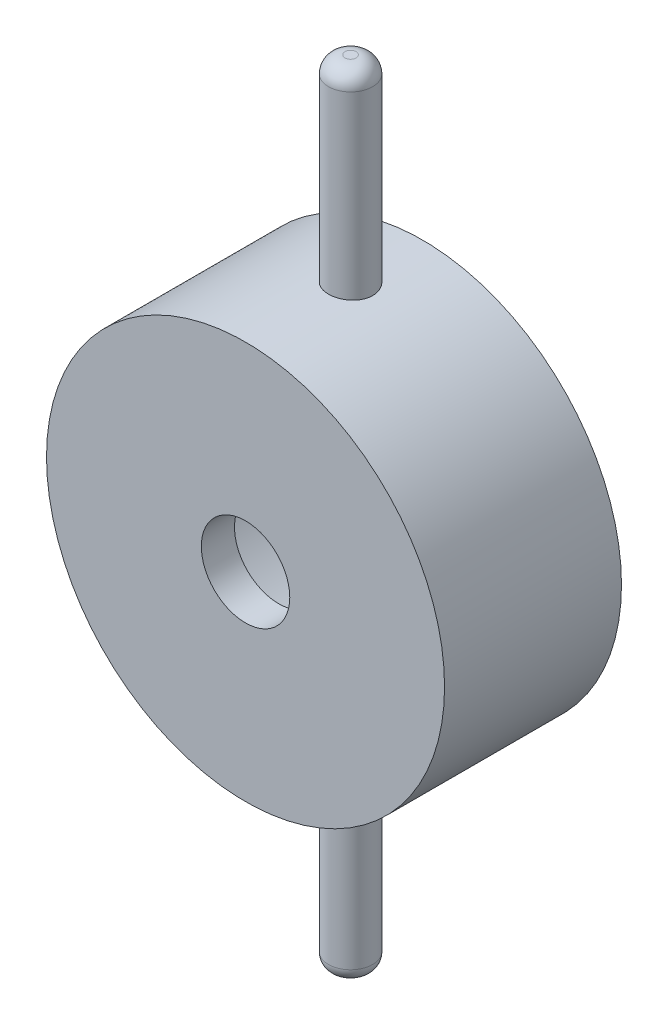
ISO-10303-21;
HEADER;
FILE_DESCRIPTION(('STEP AP214'),'2;1');
FILE_NAME('part.step','',(''),(''),'','','');
FILE_SCHEMA(('AUTOMOTIVE_DESIGN { 1 0 10303 214 1 1 1 1 }'));
ENDSEC;
DATA;
#1=APPLICATION_CONTEXT('core data for automotive mechanical design processes');
#2=APPLICATION_PROTOCOL_DEFINITION('international standard','automotive_design',2000,#1);
#3=PRODUCT_CONTEXT('',#1,'mechanical');
#4=PRODUCT('Part','Part','',(#3));
#5=PRODUCT_RELATED_PRODUCT_CATEGORY('part','',(#4));
#6=PRODUCT_DEFINITION_FORMATION('','',#4);
#7=PRODUCT_DEFINITION_CONTEXT('part definition',#1,'design');
#8=PRODUCT_DEFINITION('design','',#6,#7);
#9=PRODUCT_DEFINITION_SHAPE('','',#8);
#10=(LENGTH_UNIT() NAMED_UNIT(*) SI_UNIT(.MILLI.,.METRE.));
#11=(NAMED_UNIT(*) PLANE_ANGLE_UNIT() SI_UNIT($,.RADIAN.));
#12=(NAMED_UNIT(*) SI_UNIT($,.STERADIAN.) SOLID_ANGLE_UNIT());
#13=UNCERTAINTY_MEASURE_WITH_UNIT(LENGTH_MEASURE(1.E-05),#10,'distance_accuracy_value','');
#14=(GEOMETRIC_REPRESENTATION_CONTEXT(3) GLOBAL_UNCERTAINTY_ASSIGNED_CONTEXT((#13)) GLOBAL_UNIT_ASSIGNED_CONTEXT((#10,
#11,#12)) REPRESENTATION_CONTEXT('',''));
#15=CARTESIAN_POINT('',(0.,0.,0.));
#16=DIRECTION('',(0.,0.,1.));
#17=DIRECTION('',(1.,0.,0.));
#18=AXIS2_PLACEMENT_3D('',#15,#16,#17);
#19=CARTESIAN_POINT('',(0.,0.,32.));
#20=DIRECTION('',(0.,0.,-1.));
#21=DIRECTION('',(-1.,0.,0.));
#22=AXIS2_PLACEMENT_3D('',#19,#20,#21);
#23=CYLINDRICAL_SURFACE('',#22,36.);
#24=CARTESIAN_POINT('',(0.,-36.,17.));
#25=CARTESIAN_POINT('',(0.223941264699037,-35.9999971710871,16.9999903743455));
#26=CARTESIAN_POINT('',(0.448027205939019,-35.9978882822096,16.9811305097902));
#27=CARTESIAN_POINT('',(0.889976947693404,-35.9896783191239,16.9061849431516));
#28=CARTESIAN_POINT('',(1.10783377823557,-35.983572942543,16.8500591218983));
#29=CARTESIAN_POINT('',(1.53086215814058,-35.9680586147846,16.7022440896357));
#30=CARTESIAN_POINT('',(1.73604164147526,-35.9586517549432,16.6105773882806));
#31=CARTESIAN_POINT('',(2.12806106019971,-35.9375839621738,16.3943287716029));
#32=CARTESIAN_POINT('',(2.31490442346979,-35.9259234517738,16.2697530246617));
#33=CARTESIAN_POINT('',(2.66581151494052,-35.9015954363711,15.9906358997437));
#34=CARTESIAN_POINT('',(2.8297831590842,-35.8889241662728,15.8359790702864));
#35=CARTESIAN_POINT('',(3.12950007420101,-35.8640335665073,15.501337047927));
#36=CARTESIAN_POINT('',(3.26524398598451,-35.8518142586257,15.3213506360829));
#37=CARTESIAN_POINT('',(3.50498603632461,-35.8291733589873,14.9405721435395));
#38=CARTESIAN_POINT('',(3.60889951084678,-35.8187565931509,14.7397264459003));
#39=CARTESIAN_POINT('',(3.78149035601591,-35.8009483607062,14.3233010786259));
#40=CARTESIAN_POINT('',(3.85016879003953,-35.7935568027999,14.107721853864));
#41=CARTESIAN_POINT('',(3.95006388985288,-35.7826708846305,13.6688960042714));
#42=CARTESIAN_POINT('',(3.98143459684434,-35.7791605034939,13.4456848498581));
#43=CARTESIAN_POINT('',(4.00630012007012,-35.7763850132246,12.9971402763398));
#44=CARTESIAN_POINT('',(3.99979615128966,-35.7771197679119,12.7718069255444));
#45=CARTESIAN_POINT('',(3.94922368855802,-35.782736882028,12.3264810500568));
#46=CARTESIAN_POINT('',(3.90532400345945,-35.7876006024619,12.1064690866508));
#47=CARTESIAN_POINT('',(3.78146922315378,-35.8008985434681,11.6769547492225));
#48=CARTESIAN_POINT('',(3.70151353860304,-35.809332822402,11.4674525470469));
#49=CARTESIAN_POINT('',(3.50763212158903,-35.8288428850078,11.0643751536738));
#50=CARTESIAN_POINT('',(3.3936321376296,-35.8399244317603,10.8708359679684));
#51=CARTESIAN_POINT('',(3.13495141327351,-35.8634757446383,10.5055726985383));
#52=CARTESIAN_POINT('',(2.99026956353588,-35.8759455609506,10.3338494039533));
#53=CARTESIAN_POINT('',(2.67339229787913,-35.9009513795857,10.0161120313828));
#54=CARTESIAN_POINT('',(2.50105121133653,-35.9134873721861,9.87024318955051));
#55=CARTESIAN_POINT('',(2.13425163992195,-35.9371491420364,9.60948323665533));
#56=CARTESIAN_POINT('',(1.93979312055407,-35.9482749170867,9.49459217390847));
#57=CARTESIAN_POINT('',(1.53417327107101,-35.9678676205184,9.29905247047048));
#58=CARTESIAN_POINT('',(1.32300800960341,-35.976333920741,9.21841191804988));
#59=CARTESIAN_POINT('',(0.890019511278724,-35.9896476900257,9.09377244991667));
#60=CARTESIAN_POINT('',(0.668196668515817,-35.99449529279,9.04977218042734));
#61=CARTESIAN_POINT('',(0.221446663788539,-36.0000082213112,8.99984819656494));
#62=CARTESIAN_POINT('',(-0.00345785778178484,-36.0006955440179,8.99372421240759));
#63=CARTESIAN_POINT('',(-0.451089977374322,-35.997869624086,9.01919958502613));
#64=CARTESIAN_POINT('',(-0.67381761178264,-35.9943564517791,9.05079831018584));
#65=CARTESIAN_POINT('',(-1.11019011884666,-35.9835381866102,9.1506558809117));
#66=CARTESIAN_POINT('',(-1.32385687712367,-35.9762428689165,9.21882023623495));
#67=CARTESIAN_POINT('',(-1.73672454025379,-35.9586780068327,9.38977655545623));
#68=CARTESIAN_POINT('',(-1.93592504958459,-35.9484083811602,9.49256946570207));
#69=CARTESIAN_POINT('',(-2.31510653023491,-35.9259871400455,9.73035658214195));
#70=CARTESIAN_POINT('',(-2.49500506278204,-35.9138279560722,9.86548152187963));
#71=CARTESIAN_POINT('',(-2.82963966960439,-35.8890143170873,10.1639105966687));
#72=CARTESIAN_POINT('',(-2.98437496031115,-35.876359846668,10.3272156089047));
#73=CARTESIAN_POINT('',(-3.26499244865632,-35.851914968072,10.6782465781321));
#74=CARTESIAN_POINT('',(-3.39074265075841,-35.840128672854,10.8660783809566));
#75=CARTESIAN_POINT('',(-3.60891112010016,-35.8188194574623,11.2603125669849));
#76=CARTESIAN_POINT('',(-3.70132993400149,-35.809296500169,11.4667146455518));
#77=CARTESIAN_POINT('',(-3.84999424202287,-35.7936189645329,11.8917889174332));
#78=CARTESIAN_POINT('',(-3.90631654962256,-35.787457237671,12.1104339714952));
#79=CARTESIAN_POINT('',(-3.98143755533594,-35.7791783914912,12.5541502954833));
#80=CARTESIAN_POINT('',(-4.00023760641309,-35.7770611263396,12.7792213334069));
#81=CARTESIAN_POINT('',(-3.99975914683357,-35.7771145169331,13.2280883101301));
#82=CARTESIAN_POINT('',(-3.98068798086116,-35.7792618241774,13.4518845013619));
#83=CARTESIAN_POINT('',(-3.9054450016096,-35.7875524591414,13.8930714766512));
#84=CARTESIAN_POINT('',(-3.84927316073427,-35.7936957898334,14.1104622559441));
#85=CARTESIAN_POINT('',(-3.70148382525128,-35.8092794902223,14.5326550210184));
#86=CARTESIAN_POINT('',(-3.60987407876389,-35.8187191391705,14.7374597472708));
#87=CARTESIAN_POINT('',(-3.39383017574505,-35.8398332240413,15.1288209868962));
#88=CARTESIAN_POINT('',(-3.26939595247519,-35.8515076645075,15.3153774631659));
#89=CARTESIAN_POINT('',(-2.99045990507415,-35.8758525588044,15.6660084922529));
#90=CARTESIAN_POINT('',(-2.83580341800636,-35.888527927148,15.8299596709519));
#91=CARTESIAN_POINT('',(-2.50112838496826,-35.9134021228346,16.1296677444216));
#92=CARTESIAN_POINT('',(-2.32110381521302,-35.925600836112,16.2654179237183));
#93=CARTESIAN_POINT('',(-1.94018897354974,-35.9481870419338,16.5052086607003));
#94=CARTESIAN_POINT('',(-1.73923689283218,-35.9585689117416,16.6091514994619));
#95=CARTESIAN_POINT('',(-1.32273699032246,-35.9762927086713,16.7816749848897));
#96=CARTESIAN_POINT('',(-1.10720567988888,-35.9836380098711,16.8502949014684));
#97=CARTESIAN_POINT('',(-0.742080478625196,-35.9926465105181,16.9333983229315));
#98=CARTESIAN_POINT('',(-0.594808269722724,-35.9953909720073,16.9583390968784));
#99=CARTESIAN_POINT('',(-0.298378779805415,-35.9990686543792,16.991643097728));
#100=CARTESIAN_POINT('',(-0.149221508955014,-36.0000018850239,17.0000064139796));
#101=CARTESIAN_POINT('',(0.,-36.,17.));
#102=B_SPLINE_CURVE_WITH_KNOTS('',3,(#24,#25,#26,#27,#28,#29,#30,#31,#32,#33,#34,#35,#36,#37,
#38,#39,#40,#41,#42,#43,#44,#45,#46,#47,#48,#49,#50,#51,#52,#53,#54,#55,#56,#57,#58,#59,#60,#61,
#62,#63,#64,#65,#66,#67,#68,#69,#70,#71,#72,#73,#74,#75,#76,#77,#78,#79,#80,#81,#82,#83,#84,#85,
#86,#87,#88,#89,#90,#91,#92,#93,#94,#95,#96,#97,#98,#99,#100,#101),.UNSPECIFIED.,.T.,.F.,(4,2,2,
2,2,2,2,2,2,2,2,2,2,2,2,2,2,2,2,2,2,2,2,2,2,2,2,2,2,2,2,2,2,2,2,2,2,2,4),(0.,0.671278828541613,
1.34328150567798,2.01485926640149,2.68631123763438,3.36039299568731,4.03450720384592,
4.71039918612456,5.38627076910675,6.05934192440493,6.73239148831025,7.40241882686268,
8.07245711756367,8.74396758666022,9.41550233919238,10.0906974506658,10.7658936152352,
11.4412491390922,12.1165797089621,12.7883364134081,13.4600818703464,14.1300997551881,
14.8001359521254,15.4729286177529,16.1457422297356,16.8215617711571,17.4973702280883,
18.1717357450427,18.8460769455389,19.5167363107972,20.1873961749054,20.8579094891852,
21.5284241667564,22.2024645893278,22.8766653369059,23.5529170457317,24.2284153057591,
24.675719109969,25.1230205033015),.UNSPECIFIED.);
#103=CARTESIAN_POINT('',(0.,-36.,17.));
#104=VERTEX_POINT('',#103);
#105=EDGE_CURVE('E54',#104,#104,#102,.T.);
#106=ORIENTED_EDGE('',*,*,#105,.T.);
#107=EDGE_LOOP('',(#106));
#108=FACE_BOUND('',#107,.T.);
#109=CARTESIAN_POINT('',(0.,0.,32.));
#110=DIRECTION('',(0.,0.,1.));
#111=DIRECTION('',(1.,0.,0.));
#112=AXIS2_PLACEMENT_3D('',#109,#110,#111);
#113=CIRCLE('',#112,36.);
#114=CARTESIAN_POINT('',(36.,0.,32.));
#115=VERTEX_POINT('',#114);
#116=EDGE_CURVE('E95',#115,#115,#113,.T.);
#117=ORIENTED_EDGE('',*,*,#116,.F.);
#118=EDGE_LOOP('',(#117));
#119=FACE_BOUND('',#118,.T.);
#120=CARTESIAN_POINT('',(0.,0.,0.));
#121=DIRECTION('',(0.,0.,1.));
#122=DIRECTION('',(1.,0.,0.));
#123=AXIS2_PLACEMENT_3D('',#120,#121,#122);
#124=CIRCLE('',#123,36.);
#125=CARTESIAN_POINT('',(36.,0.,0.));
#126=VERTEX_POINT('',#125);
#127=EDGE_CURVE('E65',#126,#126,#124,.T.);
#128=ORIENTED_EDGE('',*,*,#127,.T.);
#129=EDGE_LOOP('',(#128));
#130=FACE_BOUND('',#129,.T.);
#131=CARTESIAN_POINT('',(0.,36.,9.));
#132=CARTESIAN_POINT('',(-0.223941264699037,35.9999971710871,9.00000962565452));
#133=CARTESIAN_POINT('',(-0.448027205939019,35.9978882822096,9.01886949020976));
#134=CARTESIAN_POINT('',(-0.889976947693403,35.9896783191239,9.09381505684837));
#135=CARTESIAN_POINT('',(-1.10783377823557,35.983572942543,9.14994087810168));
#136=CARTESIAN_POINT('',(-1.53086215814058,35.9680586147846,9.29775591036431));
#137=CARTESIAN_POINT('',(-1.73604164147526,35.9586517549432,9.38942261171939));
#138=CARTESIAN_POINT('',(-2.12806106019971,35.9375839621738,9.60567122839708));
#139=CARTESIAN_POINT('',(-2.31490442346979,35.9259234517738,9.73024697533831));
#140=CARTESIAN_POINT('',(-2.66581151494052,35.9015954363711,10.0093641002563));
#141=CARTESIAN_POINT('',(-2.8297831590842,35.8889241662728,10.1640209297136));
#142=CARTESIAN_POINT('',(-3.12950007420101,35.8640335665073,10.498662952073));
#143=CARTESIAN_POINT('',(-3.26524398598451,35.8518142586257,10.6786493639171));
#144=CARTESIAN_POINT('',(-3.5049860363246,35.8291733589873,11.0594278564605));
#145=CARTESIAN_POINT('',(-3.60889951084678,35.8187565931509,11.2602735540997));
#146=CARTESIAN_POINT('',(-3.78149035601591,35.8009483607062,11.6766989213741));
#147=CARTESIAN_POINT('',(-3.85016879003952,35.7935568027999,11.892278146136));
#148=CARTESIAN_POINT('',(-3.95006388985288,35.7826708846305,12.3311039957286));
#149=CARTESIAN_POINT('',(-3.98143459684434,35.7791605034939,12.5543151501419));
#150=CARTESIAN_POINT('',(-4.00630012007012,35.7763850132246,13.0028597236602));
#151=CARTESIAN_POINT('',(-3.99979615128966,35.7771197679119,13.2281930744555));
#152=CARTESIAN_POINT('',(-3.94922368855802,35.782736882028,13.6735189499432));
#153=CARTESIAN_POINT('',(-3.90532400345945,35.7876006024619,13.8935309133492));
#154=CARTESIAN_POINT('',(-3.78146922315378,35.8008985434681,14.3230452507775));
#155=CARTESIAN_POINT('',(-3.70151353860304,35.809332822402,14.5325474529531));
#156=CARTESIAN_POINT('',(-3.50763212158903,35.8288428850078,14.9356248463262));
#157=CARTESIAN_POINT('',(-3.3936321376296,35.8399244317603,15.1291640320316));
#158=CARTESIAN_POINT('',(-3.1349514132735,35.8634757446383,15.4944273014617));
#159=CARTESIAN_POINT('',(-2.99026956353588,35.8759455609506,15.6661505960467));
#160=CARTESIAN_POINT('',(-2.67339229787913,35.9009513795857,15.9838879686172));
#161=CARTESIAN_POINT('',(-2.50105121133653,35.9134873721861,16.1297568104495));
#162=CARTESIAN_POINT('',(-2.13425163992195,35.9371491420364,16.3905167633447));
#163=CARTESIAN_POINT('',(-1.93979312055407,35.9482749170867,16.5054078260915));
#164=CARTESIAN_POINT('',(-1.53417327107101,35.9678676205184,16.7009475295295));
#165=CARTESIAN_POINT('',(-1.32300800960341,35.976333920741,16.7815880819501));
#166=CARTESIAN_POINT('',(-0.890019511278724,35.9896476900257,16.9062275500833));
#167=CARTESIAN_POINT('',(-0.668196668515818,35.99449529279,16.9502278195727));
#168=CARTESIAN_POINT('',(-0.22144666378854,36.0000082213112,17.0001518034351));
#169=CARTESIAN_POINT('',(0.00345785778178408,36.0006955440179,17.0062757875924));
#170=CARTESIAN_POINT('',(0.451089977374321,35.997869624086,16.9808004149739));
#171=CARTESIAN_POINT('',(0.673817611782639,35.9943564517791,16.9492016898142));
#172=CARTESIAN_POINT('',(1.11019011884666,35.9835381866102,16.8493441190883));
#173=CARTESIAN_POINT('',(1.32385687712367,35.9762428689165,16.781179763765));
#174=CARTESIAN_POINT('',(1.73672454025379,35.9586780068327,16.6102234445438));
#175=CARTESIAN_POINT('',(1.93592504958458,35.9484083811602,16.5074305342979));
#176=CARTESIAN_POINT('',(2.31510653023491,35.9259871400455,16.269643417858));
#177=CARTESIAN_POINT('',(2.49500506278204,35.9138279560722,16.1345184781204));
#178=CARTESIAN_POINT('',(2.82963966960439,35.8890143170873,15.8360894033313));
#179=CARTESIAN_POINT('',(2.98437496031115,35.876359846668,15.6727843910953));
#180=CARTESIAN_POINT('',(3.26499244865632,35.851914968072,15.3217534218679));
#181=CARTESIAN_POINT('',(3.39074265075841,35.840128672854,15.1339216190434));
#182=CARTESIAN_POINT('',(3.60891112010016,35.8188194574623,14.7396874330151));
#183=CARTESIAN_POINT('',(3.70132993400149,35.809296500169,14.5332853544482));
#184=CARTESIAN_POINT('',(3.84999424202287,35.7936189645329,14.1082110825668));
#185=CARTESIAN_POINT('',(3.90631654962256,35.787457237671,13.8895660285048));
#186=CARTESIAN_POINT('',(3.98143755533594,35.7791783914912,13.4458497045167));
#187=CARTESIAN_POINT('',(4.00023760641309,35.7770611263396,13.2207786665931));
#188=CARTESIAN_POINT('',(3.99975914683357,35.7771145169331,12.7719116898699));
#189=CARTESIAN_POINT('',(3.98068798086116,35.7792618241774,12.5481154986381));
#190=CARTESIAN_POINT('',(3.9054450016096,35.7875524591414,12.1069285233488));
#191=CARTESIAN_POINT('',(3.84927316073427,35.7936957898334,11.8895377440559));
#192=CARTESIAN_POINT('',(3.70148382525128,35.8092794902223,11.4673449789816));
#193=CARTESIAN_POINT('',(3.60987407876389,35.8187191391705,11.2625402527292));
#194=CARTESIAN_POINT('',(3.39383017574505,35.8398332240413,10.8711790131038));
#195=CARTESIAN_POINT('',(3.26939595247519,35.8515076645075,10.6846225368341));
#196=CARTESIAN_POINT('',(2.99045990507415,35.8758525588044,10.3339915077471));
#197=CARTESIAN_POINT('',(2.83580341800636,35.888527927148,10.1700403290481));
#198=CARTESIAN_POINT('',(2.50112838496826,35.9134021228346,9.8703322555784));
#199=CARTESIAN_POINT('',(2.32110381521302,35.925600836112,9.73458207628167));
#200=CARTESIAN_POINT('',(1.94018897354974,35.9481870419338,9.49479133929974));
#201=CARTESIAN_POINT('',(1.73923689283218,35.9585689117416,9.39084850053812));
#202=CARTESIAN_POINT('',(1.32273699032246,35.9762927086713,9.21832501511034));
#203=CARTESIAN_POINT('',(1.10720567988888,35.9836380098711,9.14970509853163));
#204=CARTESIAN_POINT('',(0.742080478625197,35.9926465105181,9.06660167706846));
#205=CARTESIAN_POINT('',(0.594808269722725,35.9953909720073,9.04166090312157));
#206=CARTESIAN_POINT('',(0.298378779805415,35.9990686543792,9.00835690227201));
#207=CARTESIAN_POINT('',(0.149221508955014,36.0000018850239,8.99999358602045));
#208=CARTESIAN_POINT('',(0.,36.,9.));
#209=B_SPLINE_CURVE_WITH_KNOTS('',3,(#131,#132,#133,#134,#135,#136,#137,#138,#139,#140,#141,
#142,#143,#144,#145,#146,#147,#148,#149,#150,#151,#152,#153,#154,#155,#156,#157,#158,#159,#160,
#161,#162,#163,#164,#165,#166,#167,#168,#169,#170,#171,#172,#173,#174,#175,#176,#177,#178,#179,
#180,#181,#182,#183,#184,#185,#186,#187,#188,#189,#190,#191,#192,#193,#194,#195,#196,#197,#198,
#199,#200,#201,#202,#203,#204,#205,#206,#207,#208),.UNSPECIFIED.,.T.,.F.,(4,2,2,2,2,2,2,2,2,2,2,
2,2,2,2,2,2,2,2,2,2,2,2,2,2,2,2,2,2,2,2,2,2,2,2,2,2,2,4),(0.,0.671278828541613,1.34328150567797,
2.01485926640149,2.68631123763438,3.3603929956873,4.03450720384592,4.71039918612456,
5.38627076910675,6.05934192440493,6.73239148831025,7.40241882686268,8.07245711756367,
8.74396758666022,9.41550233919238,10.0906974506658,10.7658936152352,11.4412491390922,
12.1165797089621,12.7883364134081,13.4600818703464,14.1300997551881,14.8001359521254,
15.4729286177529,16.1457422297356,16.8215617711571,17.4973702280883,18.1717357450427,
18.8460769455388,19.5167363107972,20.1873961749054,20.8579094891852,21.5284241667564,
22.2024645893278,22.8766653369059,23.5529170457317,24.2284153057591,24.675719109969,
25.1230205033015),.UNSPECIFIED.);
#210=CARTESIAN_POINT('',(0.,36.,9.));
#211=VERTEX_POINT('',#210);
#212=EDGE_CURVE('E86',#211,#211,#209,.T.);
#213=ORIENTED_EDGE('',*,*,#212,.F.);
#214=EDGE_LOOP('',(#213));
#215=FACE_BOUND('',#214,.T.);
#216=ADVANCED_FACE('F40',(#108,#119,#130,#215),#23,.T.);
#217=CARTESIAN_POINT('',(0.,0.,32.));
#218=DIRECTION('',(0.,0.,1.));
#219=DIRECTION('',(1.,0.,0.));
#220=AXIS2_PLACEMENT_3D('',#217,#218,#219);
#221=PLANE('',#220);
#222=CARTESIAN_POINT('',(0.,0.,32.));
#223=DIRECTION('',(0.,0.,1.));
#224=DIRECTION('',(1.,0.,0.));
#225=AXIS2_PLACEMENT_3D('',#222,#223,#224);
#226=CIRCLE('',#225,8.);
#227=CARTESIAN_POINT('',(8.,0.,32.));
#228=VERTEX_POINT('',#227);
#229=EDGE_CURVE('E132',#228,#228,#226,.T.);
#230=ORIENTED_EDGE('',*,*,#229,.F.);
#231=EDGE_LOOP('',(#230));
#232=FACE_BOUND('',#231,.T.);
#233=ORIENTED_EDGE('',*,*,#116,.T.);
#234=EDGE_LOOP('',(#233));
#235=FACE_BOUND('',#234,.T.);
#236=ADVANCED_FACE('F83',(#232,#235),#221,.T.);
#237=CARTESIAN_POINT('',(0.,0.,0.));
#238=DIRECTION('',(0.,0.,1.));
#239=DIRECTION('',(1.,0.,0.));
#240=AXIS2_PLACEMENT_3D('',#237,#238,#239);
#241=PLANE('',#240);
#242=CARTESIAN_POINT('',(0.,0.,0.));
#243=DIRECTION('',(0.,0.,-1.));
#244=DIRECTION('',(-1.,0.,0.));
#245=AXIS2_PLACEMENT_3D('',#242,#243,#244);
#246=CIRCLE('',#245,28.);
#247=CARTESIAN_POINT('',(-28.,0.,0.));
#248=VERTEX_POINT('',#247);
#249=EDGE_CURVE('E134',#248,#248,#246,.T.);
#250=ORIENTED_EDGE('',*,*,#249,.F.);
#251=EDGE_LOOP('',(#250));
#252=FACE_BOUND('',#251,.T.);
#253=ORIENTED_EDGE('',*,*,#127,.F.);
#254=EDGE_LOOP('',(#253));
#255=FACE_BOUND('',#254,.T.);
#256=ADVANCED_FACE('F84',(#252,#255),#241,.F.);
#257=CARTESIAN_POINT('',(0.,71.5,13.));
#258=DIRECTION('',(0.,-1.,0.));
#259=DIRECTION('',(0.,0.,-1.));
#260=AXIS2_PLACEMENT_3D('',#257,#258,#259);
#261=CYLINDRICAL_SURFACE('',#260,4.);
#262=CARTESIAN_POINT('',(0.,68.5,13.));
#263=DIRECTION('',(0.,1.,0.));
#264=DIRECTION('',(0.,0.,1.));
#265=AXIS2_PLACEMENT_3D('',#262,#263,#264);
#266=CIRCLE('',#265,4.);
#267=CARTESIAN_POINT('',(0.,68.5,17.));
#268=VERTEX_POINT('',#267);
#269=EDGE_CURVE('E48',#268,#268,#266,.F.);
#270=ORIENTED_EDGE('',*,*,#269,.T.);
#271=EDGE_LOOP('',(#270));
#272=FACE_BOUND('',#271,.T.);
#273=ORIENTED_EDGE('',*,*,#212,.T.);
#274=EDGE_LOOP('',(#273));
#275=FACE_BOUND('',#274,.T.);
#276=ADVANCED_FACE('F76',(#272,#275),#261,.T.);
#277=CARTESIAN_POINT('',(0.,71.5,13.));
#278=DIRECTION('',(0.,1.,0.));
#279=DIRECTION('',(0.,0.,1.));
#280=AXIS2_PLACEMENT_3D('',#277,#278,#279);
#281=PLANE('',#280);
#282=CARTESIAN_POINT('',(0.,71.5,13.));
#283=DIRECTION('',(0.,1.,0.));
#284=DIRECTION('',(0.,0.,1.));
#285=AXIS2_PLACEMENT_3D('',#282,#283,#284);
#286=CIRCLE('',#285,1.);
#287=CARTESIAN_POINT('',(0.,71.5,14.));
#288=VERTEX_POINT('',#287);
#289=EDGE_CURVE('E55',#288,#288,#286,.T.);
#290=ORIENTED_EDGE('',*,*,#289,.T.);
#291=EDGE_LOOP('',(#290));
#292=FACE_BOUND('',#291,.T.);
#293=ADVANCED_FACE('F72',(#292),#281,.T.);
#294=CARTESIAN_POINT('',(0.,68.5,13.));
#295=DIRECTION('',(0.,1.,0.));
#296=DIRECTION('',(0.,0.,1.));
#297=AXIS2_PLACEMENT_3D('',#294,#295,#296);
#298=DEGENERATE_TOROIDAL_SURFACE('',#297,1.,3.,.T.);
#299=ORIENTED_EDGE('',*,*,#269,.F.);
#300=EDGE_LOOP('',(#299));
#301=FACE_BOUND('',#300,.T.);
#302=ORIENTED_EDGE('',*,*,#289,.F.);
#303=EDGE_LOOP('',(#302));
#304=FACE_BOUND('',#303,.T.);
#305=ADVANCED_FACE('F75',(#301,#304),#298,.T.);
#306=CARTESIAN_POINT('',(0.,-71.5,13.));
#307=DIRECTION('',(0.,1.,0.));
#308=DIRECTION('',(0.,0.,1.));
#309=AXIS2_PLACEMENT_3D('',#306,#307,#308);
#310=CYLINDRICAL_SURFACE('',#309,4.);
#311=CARTESIAN_POINT('',(0.,-69.,13.));
#312=DIRECTION('',(0.,-1.,0.));
#313=DIRECTION('',(0.,0.,-1.));
#314=AXIS2_PLACEMENT_3D('',#311,#312,#313);
#315=CIRCLE('',#314,4.);
#316=CARTESIAN_POINT('',(0.,-69.,9.));
#317=VERTEX_POINT('',#316);
#318=EDGE_CURVE('E42',#317,#317,#315,.F.);
#319=ORIENTED_EDGE('',*,*,#318,.T.);
#320=EDGE_LOOP('',(#319));
#321=FACE_BOUND('',#320,.T.);
#322=ORIENTED_EDGE('',*,*,#105,.F.);
#323=EDGE_LOOP('',(#322));
#324=FACE_BOUND('',#323,.T.);
#325=ADVANCED_FACE('F66',(#321,#324),#310,.T.);
#326=CARTESIAN_POINT('',(0.,-71.5,13.));
#327=DIRECTION('',(0.,-1.,0.));
#328=DIRECTION('',(0.,0.,1.));
#329=AXIS2_PLACEMENT_3D('',#326,#327,#328);
#330=PLANE('',#329);
#331=CARTESIAN_POINT('',(0.,-71.5,13.));
#332=DIRECTION('',(0.,-1.,0.));
#333=DIRECTION('',(0.,0.,-1.));
#334=AXIS2_PLACEMENT_3D('',#331,#332,#333);
#335=CIRCLE('',#334,1.5);
#336=CARTESIAN_POINT('',(0.,-71.5,11.5));
#337=VERTEX_POINT('',#336);
#338=EDGE_CURVE('E10',#337,#337,#335,.T.);
#339=ORIENTED_EDGE('',*,*,#338,.T.);
#340=EDGE_LOOP('',(#339));
#341=FACE_BOUND('',#340,.T.);
#342=ADVANCED_FACE('F71',(#341),#330,.T.);
#343=CARTESIAN_POINT('',(0.,0.,26.));
#344=DIRECTION('',(0.,0.,1.));
#345=DIRECTION('',(1.,0.,0.));
#346=AXIS2_PLACEMENT_3D('',#343,#344,#345);
#347=PLANE('',#346);
#348=CARTESIAN_POINT('',(0.,0.,26.));
#349=DIRECTION('',(0.,0.,1.));
#350=DIRECTION('',(1.,0.,0.));
#351=AXIS2_PLACEMENT_3D('',#348,#349,#350);
#352=CIRCLE('',#351,8.);
#353=CARTESIAN_POINT('',(8.,0.,26.));
#354=VERTEX_POINT('',#353);
#355=EDGE_CURVE('E133',#354,#354,#352,.T.);
#356=ORIENTED_EDGE('',*,*,#355,.T.);
#357=EDGE_LOOP('',(#356));
#358=FACE_BOUND('',#357,.T.);
#359=CARTESIAN_POINT('',(0.,0.,26.));
#360=DIRECTION('',(0.,0.,-1.));
#361=DIRECTION('',(-1.,0.,0.));
#362=AXIS2_PLACEMENT_3D('',#359,#360,#361);
#363=CIRCLE('',#362,9.99999999999999);
#364=CARTESIAN_POINT('',(-9.99999999999999,0.,26.));
#365=VERTEX_POINT('',#364);
#366=EDGE_CURVE('E64',#365,#365,#363,.T.);
#367=ORIENTED_EDGE('',*,*,#366,.T.);
#368=EDGE_LOOP('',(#367));
#369=FACE_BOUND('',#368,.T.);
#370=ADVANCED_FACE('F142',(#358,#369),#347,.F.);
#371=CARTESIAN_POINT('',(0.,0.,-9.53547678038324));
#372=DIRECTION('',(0.,0.,-1.));
#373=DIRECTION('',(-1.,0.,0.));
#374=AXIS2_PLACEMENT_3D('',#371,#372,#373);
#375=CYLINDRICAL_SURFACE('',#374,9.99999999999999);
#376=ORIENTED_EDGE('',*,*,#366,.F.);
#377=EDGE_LOOP('',(#376));
#378=FACE_BOUND('',#377,.T.);
#379=CARTESIAN_POINT('',(0.,0.,28.));
#380=DIRECTION('',(0.,0.,-1.));
#381=DIRECTION('',(-1.,0.,0.));
#382=AXIS2_PLACEMENT_3D('',#379,#380,#381);
#383=CIRCLE('',#382,9.99999999999999);
#384=CARTESIAN_POINT('',(-9.99999999999999,0.,28.));
#385=VERTEX_POINT('',#384);
#386=EDGE_CURVE('E123',#385,#385,#383,.T.);
#387=ORIENTED_EDGE('',*,*,#386,.T.);
#388=EDGE_LOOP('',(#387));
#389=FACE_BOUND('',#388,.T.);
#390=ADVANCED_FACE('F162',(#378,#389),#375,.T.);
#391=CARTESIAN_POINT('',(-9.99999999999999,0.,28.));
#392=DIRECTION('',(0.,0.,1.));
#393=DIRECTION('',(1.,0.,0.));
#394=AXIS2_PLACEMENT_3D('',#391,#392,#393);
#395=PLANE('',#394);
#396=ORIENTED_EDGE('',*,*,#386,.F.);
#397=EDGE_LOOP('',(#396));
#398=FACE_BOUND('',#397,.T.);
#399=CARTESIAN_POINT('',(0.,0.,28.));
#400=DIRECTION('',(0.,0.,-1.));
#401=DIRECTION('',(-1.,0.,0.));
#402=AXIS2_PLACEMENT_3D('',#399,#400,#401);
#403=CIRCLE('',#402,28.);
#404=CARTESIAN_POINT('',(-28.,0.,28.));
#405=VERTEX_POINT('',#404);
#406=EDGE_CURVE('E129',#405,#405,#403,.T.);
#407=ORIENTED_EDGE('',*,*,#406,.T.);
#408=EDGE_LOOP('',(#407));
#409=FACE_BOUND('',#408,.T.);
#410=ADVANCED_FACE('F159',(#398,#409),#395,.F.);
#411=CARTESIAN_POINT('',(0.,0.,-9.53547678038324));
#412=DIRECTION('',(0.,0.,-1.));
#413=DIRECTION('',(-1.,0.,0.));
#414=AXIS2_PLACEMENT_3D('',#411,#412,#413);
#415=CYLINDRICAL_SURFACE('',#414,28.);
#416=ORIENTED_EDGE('',*,*,#406,.F.);
#417=EDGE_LOOP('',(#416));
#418=FACE_BOUND('',#417,.T.);
#419=ORIENTED_EDGE('',*,*,#249,.T.);
#420=EDGE_LOOP('',(#419));
#421=FACE_BOUND('',#420,.T.);
#422=ADVANCED_FACE('F150',(#418,#421),#415,.F.);
#423=CARTESIAN_POINT('',(0.,0.,26.));
#424=DIRECTION('',(0.,0.,1.));
#425=DIRECTION('',(1.,0.,0.));
#426=AXIS2_PLACEMENT_3D('',#423,#424,#425);
#427=CYLINDRICAL_SURFACE('',#426,8.);
#428=ORIENTED_EDGE('',*,*,#355,.F.);
#429=EDGE_LOOP('',(#428));
#430=FACE_BOUND('',#429,.T.);
#431=ORIENTED_EDGE('',*,*,#229,.T.);
#432=EDGE_LOOP('',(#431));
#433=FACE_BOUND('',#432,.T.);
#434=ADVANCED_FACE('F144',(#430,#433),#427,.F.);
#435=CARTESIAN_POINT('',(0.,-69.,13.));
#436=DIRECTION('',(0.,-1.,0.));
#437=DIRECTION('',(0.,0.,-1.));
#438=AXIS2_PLACEMENT_3D('',#435,#436,#437);
#439=DEGENERATE_TOROIDAL_SURFACE('',#438,1.5,2.5,.T.);
#440=ORIENTED_EDGE('',*,*,#338,.F.);
#441=EDGE_LOOP('',(#440));
#442=FACE_BOUND('',#441,.T.);
#443=ORIENTED_EDGE('',*,*,#318,.F.);
#444=EDGE_LOOP('',(#443));
#445=FACE_BOUND('',#444,.T.);
#446=ADVANCED_FACE('F39',(#442,#445),#439,.T.);
#447=CLOSED_SHELL('',(#216,#236,#256,#276,#293,#305,#325,#342,#370,#390,#410,#422,#434,#446));
#448=MANIFOLD_SOLID_BREP('B2',#447);
#449=ADVANCED_BREP_SHAPE_REPRESENTATION('',(#18,#448),#14);
#450=SHAPE_DEFINITION_REPRESENTATION(#9,#449);
ENDSEC;
END-ISO-10303-21;
